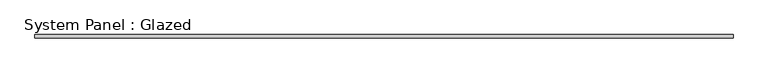
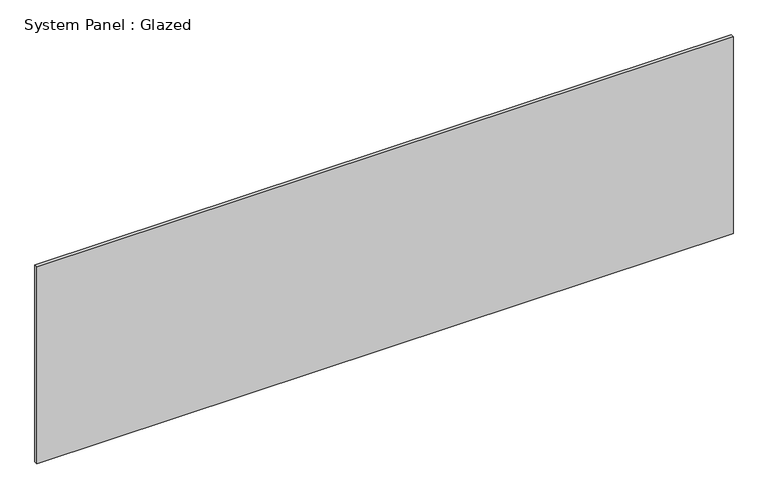
"""IFC4 building model written with IfcOpenShell, lengths in millimetres: plate geometry, System Panel : Glazed."""

from ifc_helpers import new_model, si_unit, origin, origin_with_axes, place, context, project, spatial, polyline, outline, extrude, source, transform, mapped, element, save


def system_panel_glazed_00b49b46(model_context):
    return source(origin(), model_context, "Body", "SweptSolid", [
        extrude(outline(polyline([(2551.6092472, 19.05), (-2551.6092472, 19.05), (-2551.6092472, 44.45), (2551.6092472, 44.45), (2551.6092472, 19.05)])), origin_with_axes(), (0.0, 0.0, 1.0), 1524.0),
    ])


if __name__ == "__main__":
    model = new_model("IFC4")
    model_context = context("Model", 3, world=origin())
    ifc_project = project(units=[si_unit("LENGTHUNIT", "METRE", prefix="MILLI")], contexts=[model_context])
    site = spatial("IfcSite", under=ifc_project)
    building = spatial("IfcBuilding", under=site)
    placement = place(None, origin())
    system_panel_glazed_shape = system_panel_glazed_00b49b46(model_context)
    element("IfcPlate", 1, ObjectType="System Panel : Glazed", at=placement, inside=building, context=model_context, shape_type="MappedRepresentation", body=[
        mapped(system_panel_glazed_shape, transform((0.0, 0.0, 0.0), x_axis=(1.0, 0.0, 0.0), y_axis=(0.0, 1.0, 0.0), z_axis=(0.0, 0.0, 1.0))),
    ])
    save(model, "model.ifc")

# Revit data of these elements
# Type "System Panel : Glazed"
#   Construction Type Id = "GSP4R"
#   Analytic Construction = "1/8 in Pilkington single glazing"
#   Visual Light Transmittance = 0.9
#   Solar Heat Gain Coefficient = 0.86
#   Heat Transfer Coefficient (U) = 1.18115 BTU/(h·ft²·°F)
# Element 1 (IfcPlate, "System Panel : Glazed")
#   Materials on its faces: "Glass"
# Materials
#   "Glass": class "Glass", colour RGB 0 128 192, transparency 0.75, Description = "Soda Lime Glass", Cost = 0
